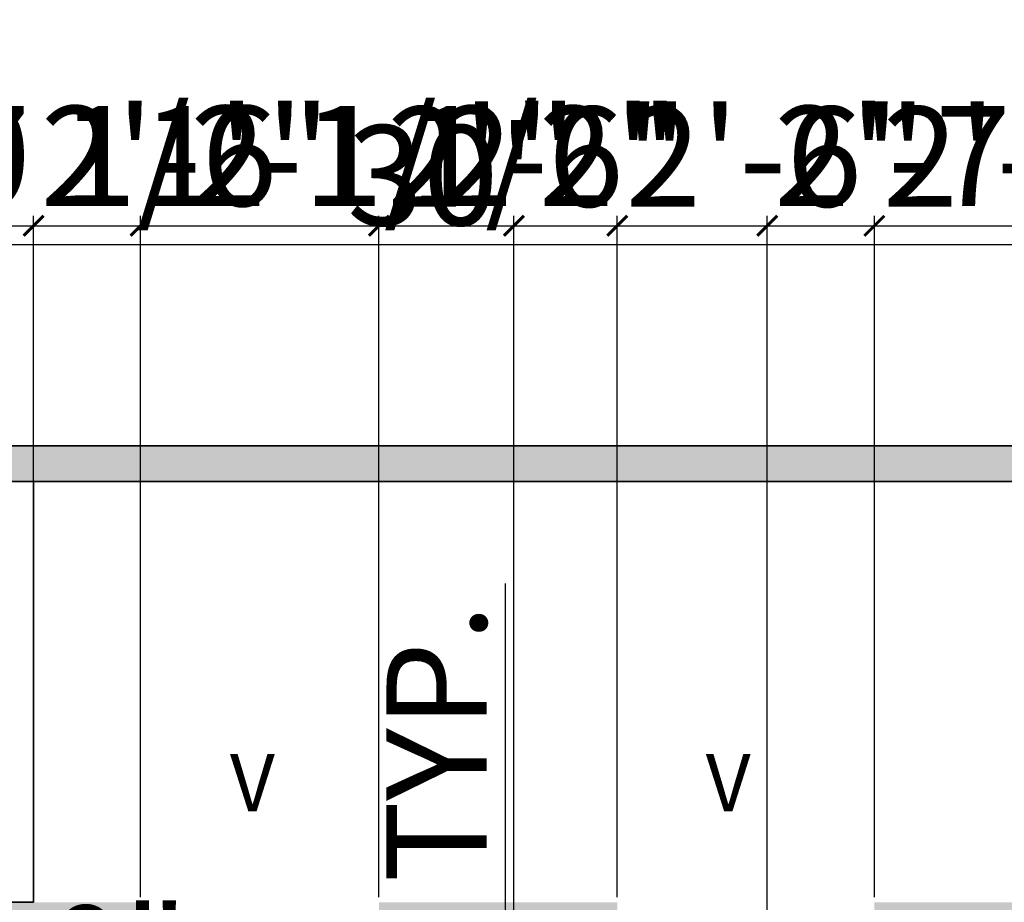
# Model space of a CAD drawing. Units: inches. Extents: x 1763 to 2368, y 1500 to 2097.
# Tile 12 of 24: x 1956 to 2079, y 1986 to 2097. Entities that reach past the tile are written whole.
import ezdxf

# ---------------------------------------------------------------- set-up
doc = ezdxf.new("R2010")
doc.units = ezdxf.units.IN
for name, color, linetype, lineweight in [('A-ANNO-DIMS', 2, 'Continuous', 18), ('A-ANNO-TEXT', 7, 'Continuous', 18), ('A-WALL', 7, 'Continuous', 35), ('A-WALL-PATT', 7, 'Continuous', 13)]:
    doc.layers.add(name, color=color, linetype=linetype, lineweight=lineweight)
doc.styles.get("Standard").update_dxf_attribs({"font": 'arial.ttf'})
doc.dimstyles.new('ISO-25', dxfattribs={"dimtxt": 12.5, "dimasz": 2.5, "dimexe": 1.25, "dimexo": 0.625, "dimtad": 1, "dimdec": 0, "dimlunit": 4, "dimtxsty": 'Standard', "dimblk": 'ARCHTICK', "dimcen": 2.5, "dimclrd": 3, "dimclrt": 4, "dimadec": 0, "dimazin": 0, "dimtfac": 1, "dimtdec": 0, "dimtmove": 0, "dimatfit": 3, "dimfxl": 1, "dimarcsym": 0})

# ---------------------------------------------------------------- blocks, each defined once
blk = doc.blocks.new('_ArchTick')
at = {"color": 0, "linetype": 'ByBlock', "const_width": 0.15}
blk.add_lwpolyline([(-0.5, -0.5), (0.5, 0.5)], dxfattribs=at)
blk = doc.blocks.new('*D21')
at = {"layer": 'A-ANNO-DIMS', "color": 0, "lineweight": -2, "transparency": 16777216}
for p, q in [((1829.09, 2043.9), (1829.09, 2069.68)), ((2189.09, 2043.9), (2189.09, 2069.68)), ((1829.09, 2068.43), (2189.09, 2068.43))]:
    blk.add_line(p, q, dxfattribs=at)
at = {"layer": 'Defpoints', "color": 0, "transparency": 16777216}
for p in [(2189.09, 2068.43), (1829.09, 2043.27), (2189.09, 2043.27)]:
    blk.add_point(p, dxfattribs=at)
at = {"layer": 'A-ANNO-DIMS', "color": 0, "lineweight": -2, "transparency": 16777216, "xscale": 2.5, "yscale": 2.5, "zscale": 2.5, "rotation": 180}
blk.add_blockref('_ArchTick', (1829.09, 2068.43), dxfattribs=at)
at = {"layer": 'A-ANNO-DIMS', "color": 0, "lineweight": -2, "transparency": 16777216, "xscale": 2.5, "yscale": 2.5, "zscale": 2.5}
blk.add_blockref('_ArchTick', (2189.09, 2068.43), dxfattribs=at)
at = {"layer": 'A-ANNO-DIMS', "color": 0, "transparency": 16777216, "insert": (2009.09, 2075.45), "char_height": 12.5, "attachment_point": 5}
blk.add_mtext("30'", dxfattribs=at)
blk = doc.blocks.new('*D35')
at = {"layer": 'A-ANNO-DIMS', "color": 0, "lineweight": -2, "transparency": 16777216}
for p, q in [((1889.68, 1972.15), (1889.68, 1969.72)), ((1901.68, 1972.15), (1901.68, 1969.72))]:
    blk.add_line(p, q, dxfattribs=at)
at = {"layer": 'A-ANNO-DIMS', "color": 3, "lineweight": -2, "transparency": 16777216}
for p, q in [((1889.68, 1970.97), (1901.68, 1970.97)), ((1901.68, 1970.97), (1977.79, 1970.97))]:
    blk.add_line(p, q, dxfattribs=at)
at = {"layer": 'Defpoints', "color": 0, "transparency": 16777216}
for p in [(1889.68, 1972.77), (1901.68, 1972.77), (1901.68, 1970.97)]:
    blk.add_point(p, dxfattribs=at)
at = {"layer": 'A-ANNO-DIMS', "color": 3, "lineweight": -2, "transparency": 16777216, "xscale": 2.5, "yscale": 2.5, "zscale": 2.5, "rotation": 180}
blk.add_blockref('_ArchTick', (1889.68, 1970.97), dxfattribs=at)
at = {"layer": 'A-ANNO-DIMS', "color": 3, "lineweight": -2, "transparency": 16777216, "xscale": 2.5, "yscale": 2.5, "zscale": 2.5}
blk.add_blockref('_ArchTick', (1901.68, 1970.97), dxfattribs=at)
at = {"layer": 'A-ANNO-DIMS', "color": 4, "transparency": 16777216, "insert": (1940.99, 1977.98), "char_height": 12.5, "attachment_point": 5}
blk.add_mtext('TAP 1\'-0"', dxfattribs=at)
blk = doc.blocks.new('*D37')
at = {"layer": 'A-ANNO-DIMS', "color": 3, "lineweight": -2, "transparency": 16777216}
for p, q in [((2017.06, 1907.01), (2017.06, 2026.09)), ((2017.06, 1900.14), (2017.06, 1907.01))]:
    blk.add_line(p, q, dxfattribs=at)
at = {"layer": 'A-ANNO-DIMS', "color": 0, "lineweight": -2, "transparency": 16777216}
for p, q in [((2017.47, 1907.01), (2015.81, 1907.01)), ((2017.47, 1900.14), (2015.81, 1900.14))]:
    blk.add_line(p, q, dxfattribs=at)
at = {"layer": 'Defpoints', "color": 0, "transparency": 16777216}
for p in [(2017.06, 1907.01), (2018.09, 1907.01), (2018.09, 1900.14)]:
    blk.add_point(p, dxfattribs=at)
at = {"layer": 'A-ANNO-DIMS', "color": 3, "lineweight": -2, "transparency": 16777216, "xscale": 2.5, "yscale": 2.5, "zscale": 2.5}
for p, rotation in [((2017.06, 1907.01), 90), ((2017.06, 1900.14), 270)]:
    blk.add_blockref('_ArchTick', p, dxfattribs=dict(at, rotation=rotation))
at = {"layer": 'A-ANNO-DIMS', "color": 4, "transparency": 16777216, "insert": (2010.05, 1967.8), "char_height": 12.5, "attachment_point": 5, "rotation": 90}
blk.add_mtext('TAP 0\'-7" TYP.', dxfattribs=at)
blk = doc.blocks.new('*D58')
at = {"layer": 'A-ANNO-DIMS', "color": 0, "lineweight": -2, "transparency": 16777216}
for p, q in [((1871.68, 1635.9), (1871.68, 2072.02)), ((1927.07, 1635.9), (1927.07, 2072.02))]:
    blk.add_line(p, q, dxfattribs=at)
at = {"layer": 'A-ANNO-DIMS', "color": 3, "lineweight": -2, "transparency": 16777216}
for p, q in [((1871.68, 2070.77), (1927.07, 2070.77)), ((1927.07, 2070.77), (1993.68, 2070.77))]:
    blk.add_line(p, q, dxfattribs=at)
at = {"layer": 'Defpoints', "color": 0, "transparency": 16777216}
for p in [(1927.07, 2070.77), (1871.68, 1635.27), (1927.07, 1635.27)]:
    blk.add_point(p, dxfattribs=at)
at = {"layer": 'A-ANNO-DIMS', "color": 3, "lineweight": -2, "transparency": 16777216, "xscale": 2.5, "yscale": 2.5, "zscale": 2.5, "rotation": 180}
blk.add_blockref('_ArchTick', (1871.68, 2070.77), dxfattribs=at)
at = {"layer": 'A-ANNO-DIMS', "color": 3, "lineweight": -2, "transparency": 16777216, "xscale": 2.5, "yscale": 2.5, "zscale": 2.5}
blk.add_blockref('_ArchTick', (1927.07, 2070.77), dxfattribs=at)
at = {"layer": 'A-ANNO-DIMS', "color": 4, "transparency": 16777216, "insert": (1961.63, 2077.86), "char_height": 12.5, "attachment_point": 5}
blk.add_mtext('4\'-7 1/2"', dxfattribs=at)
blk = doc.blocks.new('*D66')
at = {"layer": 'A-ANNO-DIMS', "color": 0, "lineweight": -2, "transparency": 16777216}
for p, q in [((1927.39, 1986.9), (1927.39, 2072.02)), ((1958.09, 1986.9), (1958.09, 2072.02))]:
    blk.add_line(p, q, dxfattribs=at)
at = {"layer": 'A-ANNO-DIMS', "color": 3, "lineweight": -2, "transparency": 16777216}
for p, q in [((1927.39, 2070.77), (1958.09, 2070.77)), ((1958.09, 2070.77), (2024.41, 2070.77))]:
    blk.add_line(p, q, dxfattribs=at)
at = {"layer": 'Defpoints', "color": 0, "transparency": 16777216}
for p in [(1958.09, 2070.77), (1927.39, 1986.27), (1958.09, 1986.27)]:
    blk.add_point(p, dxfattribs=at)
at = {"layer": 'A-ANNO-DIMS', "color": 3, "lineweight": -2, "transparency": 16777216, "xscale": 2.5, "yscale": 2.5, "zscale": 2.5, "rotation": 180}
blk.add_blockref('_ArchTick', (1927.39, 2070.77), dxfattribs=at)
at = {"layer": 'A-ANNO-DIMS', "color": 3, "lineweight": -2, "transparency": 16777216, "xscale": 2.5, "yscale": 2.5, "zscale": 2.5}
blk.add_blockref('_ArchTick', (1958.09, 2070.77), dxfattribs=at)
at = {"layer": 'A-ANNO-DIMS', "color": 4, "transparency": 16777216, "insert": (1992.5, 2077.86), "char_height": 12.5, "attachment_point": 5}
blk.add_mtext('2\'-6 1/2"', dxfattribs=at)
blk = doc.blocks.new('*D67')
at = {"layer": 'A-ANNO-DIMS', "color": 0, "lineweight": -2, "transparency": 16777216}
for p, q in [((1890.93, 1986.9), (1890.93, 2072.02)), ((1927.39, 1986.9), (1927.39, 2072.02))]:
    blk.add_line(p, q, dxfattribs=at)
at = {"layer": 'A-ANNO-DIMS', "color": 3, "lineweight": -2, "transparency": 16777216}
for p, q in [((1890.93, 2070.77), (1927.39, 2070.77)), ((1927.39, 2070.77), (1993.49, 2070.77))]:
    blk.add_line(p, q, dxfattribs=at)
at = {"layer": 'Defpoints', "color": 0, "transparency": 16777216}
for p in [(1927.39, 2070.77), (1890.93, 1986.27), (1927.39, 1986.27)]:
    blk.add_point(p, dxfattribs=at)
at = {"layer": 'A-ANNO-DIMS', "color": 3, "lineweight": -2, "transparency": 16777216, "xscale": 2.5, "yscale": 2.5, "zscale": 2.5, "rotation": 180}
blk.add_blockref('_ArchTick', (1890.93, 2070.77), dxfattribs=at)
at = {"layer": 'A-ANNO-DIMS', "color": 3, "lineweight": -2, "transparency": 16777216, "xscale": 2.5, "yscale": 2.5, "zscale": 2.5}
blk.add_blockref('_ArchTick', (1927.39, 2070.77), dxfattribs=at)
at = {"layer": 'A-ANNO-DIMS', "color": 4, "transparency": 16777216, "insert": (1961.69, 2077.87), "char_height": 12.5, "attachment_point": 5}
blk.add_mtext('3\'-0 1/2"', dxfattribs=at)
blk = doc.blocks.new('*D72')
at = {"layer": 'A-ANNO-DIMS', "color": 0, "lineweight": -2, "transparency": 16777216}
for p, q in [((2018.09, 1885.9), (2018.09, 2072.02)), ((2049.74, 1885.9), (2049.74, 2072.02))]:
    blk.add_line(p, q, dxfattribs=at)
at = {"layer": 'A-ANNO-DIMS', "color": 3, "lineweight": -2, "transparency": 16777216}
for p, q in [((2018.09, 2070.77), (2049.74, 2070.77)), ((2049.74, 2070.77), (2116.06, 2070.77))]:
    blk.add_line(p, q, dxfattribs=at)
at = {"layer": 'Defpoints', "color": 0, "transparency": 16777216}
for p in [(2049.74, 2070.77), (2018.09, 1885.27), (2049.74, 1885.27)]:
    blk.add_point(p, dxfattribs=at)
at = {"layer": 'A-ANNO-DIMS', "color": 3, "lineweight": -2, "transparency": 16777216, "xscale": 2.5, "yscale": 2.5, "zscale": 2.5, "rotation": 180}
blk.add_blockref('_ArchTick', (2018.09, 2070.77), dxfattribs=at)
at = {"layer": 'A-ANNO-DIMS', "color": 3, "lineweight": -2, "transparency": 16777216, "xscale": 2.5, "yscale": 2.5, "zscale": 2.5}
blk.add_blockref('_ArchTick', (2049.74, 2070.77), dxfattribs=at)
at = {"layer": 'A-ANNO-DIMS', "color": 4, "transparency": 16777216, "insert": (2084.15, 2077.86), "char_height": 12.5, "attachment_point": 5}
blk.add_mtext('2\'-7 1/2"', dxfattribs=at)
blk = doc.blocks.new('*D73')
at = {"layer": 'A-ANNO-DIMS', "color": 0, "lineweight": -2, "transparency": 16777216}
for p, q in [((1958.09, 1986.9), (1958.09, 2072.02)), ((1971.46, 1986.9), (1971.46, 2072.02))]:
    blk.add_line(p, q, dxfattribs=at)
at = {"layer": 'A-ANNO-DIMS', "color": 3, "lineweight": -2, "transparency": 16777216}
for p, q in [((1958.09, 2070.77), (1971.46, 2070.77)), ((1971.46, 2070.77), (2036.38, 2070.77))]:
    blk.add_line(p, q, dxfattribs=at)
at = {"layer": 'Defpoints', "color": 0, "transparency": 16777216}
for p in [(1971.46, 2070.77), (1958.09, 1986.27), (1971.46, 1986.27)]:
    blk.add_point(p, dxfattribs=at)
at = {"layer": 'A-ANNO-DIMS', "color": 3, "lineweight": -2, "transparency": 16777216, "xscale": 2.5, "yscale": 2.5, "zscale": 2.5, "rotation": 180}
blk.add_blockref('_ArchTick', (1958.09, 2070.77), dxfattribs=at)
at = {"layer": 'A-ANNO-DIMS', "color": 3, "lineweight": -2, "transparency": 16777216, "xscale": 2.5, "yscale": 2.5, "zscale": 2.5}
blk.add_blockref('_ArchTick', (1971.46, 2070.77), dxfattribs=at)
at = {"layer": 'A-ANNO-DIMS', "color": 4, "transparency": 16777216, "insert": (2005.17, 2077.86), "char_height": 12.5, "attachment_point": 5}
blk.add_mtext('1\'-1 1/2"', dxfattribs=at)
blk = doc.blocks.new('*D74')
at = {"layer": 'A-ANNO-DIMS', "color": 0, "lineweight": -2, "transparency": 16777216}
for p, q in [((1971.46, 1986.9), (1971.46, 2072.02)), ((2001.23, 1986.9), (2001.23, 2072.02))]:
    blk.add_line(p, q, dxfattribs=at)
at = {"layer": 'A-ANNO-DIMS', "color": 3, "lineweight": -2, "transparency": 16777216}
for p, q in [((1971.46, 2070.77), (2001.23, 2070.77)), ((2001.23, 2070.77), (2038.42, 2070.77))]:
    blk.add_line(p, q, dxfattribs=at)
at = {"layer": 'Defpoints', "color": 0, "transparency": 16777216}
for p in [(2001.23, 2070.77), (1971.46, 1986.27), (2001.23, 1986.27)]:
    blk.add_point(p, dxfattribs=at)
at = {"layer": 'A-ANNO-DIMS', "color": 3, "lineweight": -2, "transparency": 16777216, "xscale": 2.5, "yscale": 2.5, "zscale": 2.5, "rotation": 180}
blk.add_blockref('_ArchTick', (1971.46, 2070.77), dxfattribs=at)
at = {"layer": 'A-ANNO-DIMS', "color": 3, "lineweight": -2, "transparency": 16777216, "xscale": 2.5, "yscale": 2.5, "zscale": 2.5}
blk.add_blockref('_ArchTick', (2001.23, 2070.77), dxfattribs=at)
at = {"layer": 'A-ANNO-DIMS', "color": 4, "transparency": 16777216, "insert": (2021.08, 2077.78), "char_height": 12.5, "attachment_point": 5}
blk.add_mtext('2\'-6"', dxfattribs=at)
blk = doc.blocks.new('*D75')
at = {"layer": 'A-ANNO-DIMS', "color": 0, "lineweight": -2, "transparency": 16777216}
for p, q in [((2001.23, 1986.9), (2001.23, 2072.02)), ((2031.02, 1986.9), (2031.02, 2072.02))]:
    blk.add_line(p, q, dxfattribs=at)
at = {"layer": 'A-ANNO-DIMS', "color": 3, "lineweight": -2, "transparency": 16777216}
for p, q in [((2001.23, 2070.77), (2031.02, 2070.77)), ((2031.02, 2070.77), (2068.21, 2070.77))]:
    blk.add_line(p, q, dxfattribs=at)
at = {"layer": 'Defpoints', "color": 0, "transparency": 16777216}
for p in [(2031.02, 2070.77), (2001.23, 1986.27), (2031.02, 1986.27)]:
    blk.add_point(p, dxfattribs=at)
at = {"layer": 'A-ANNO-DIMS', "color": 3, "lineweight": -2, "transparency": 16777216, "xscale": 2.5, "yscale": 2.5, "zscale": 2.5, "rotation": 180}
blk.add_blockref('_ArchTick', (2001.23, 2070.77), dxfattribs=at)
at = {"layer": 'A-ANNO-DIMS', "color": 3, "lineweight": -2, "transparency": 16777216, "xscale": 2.5, "yscale": 2.5, "zscale": 2.5}
blk.add_blockref('_ArchTick', (2031.02, 2070.77), dxfattribs=at)
at = {"layer": 'A-ANNO-DIMS', "color": 4, "transparency": 16777216, "insert": (2050.86, 2077.78), "char_height": 12.5, "attachment_point": 5}
blk.add_mtext('2\'-6"', dxfattribs=at)
blk = doc.blocks.new('*D76')
at = {"layer": 'A-ANNO-DIMS', "color": 0, "lineweight": -2, "transparency": 16777216}
for p, q in [((2031.02, 1986.9), (2031.02, 2072.02)), ((2063.14, 1986.9), (2063.14, 2072.02))]:
    blk.add_line(p, q, dxfattribs=at)
at = {"layer": 'A-ANNO-DIMS', "color": 3, "lineweight": -2, "transparency": 16777216}
for p, q in [((2031.02, 2070.77), (2063.14, 2070.77)), ((2063.14, 2070.77), (2100.33, 2070.77))]:
    blk.add_line(p, q, dxfattribs=at)
at = {"layer": 'Defpoints', "color": 0, "transparency": 16777216}
for p in [(2063.14, 2070.77), (2031.02, 1986.27), (2063.14, 1986.27)]:
    blk.add_point(p, dxfattribs=at)
at = {"layer": 'A-ANNO-DIMS', "color": 3, "lineweight": -2, "transparency": 16777216, "xscale": 2.5, "yscale": 2.5, "zscale": 2.5, "rotation": 180}
blk.add_blockref('_ArchTick', (2031.02, 2070.77), dxfattribs=at)
at = {"layer": 'A-ANNO-DIMS', "color": 3, "lineweight": -2, "transparency": 16777216, "xscale": 2.5, "yscale": 2.5, "zscale": 2.5}
blk.add_blockref('_ArchTick', (2063.14, 2070.77), dxfattribs=at)
at = {"layer": 'A-ANNO-DIMS', "color": 4, "transparency": 16777216, "insert": (2082.99, 2077.78), "char_height": 12.5, "attachment_point": 5}
blk.add_mtext('2\'-8"', dxfattribs=at)
blk = doc.blocks.new('*D84')
at = {"layer": 'A-ANNO-DIMS', "color": 0, "lineweight": -2, "transparency": 16777216}
for p, q in [((1829.09, 2043.9), (1829.09, 2072.02)), ((1958.09, 2039.45), (1958.09, 2072.02))]:
    blk.add_line(p, q, dxfattribs=at)
at = {"layer": 'A-ANNO-DIMS', "color": 3, "lineweight": -2, "transparency": 16777216}
blk.add_line((1829.09, 2070.77), (1958.09, 2070.77), dxfattribs=at)
at = {"layer": 'Defpoints', "color": 0, "transparency": 16777216}
for p in [(1958.09, 2070.77), (1829.09, 2043.27), (1958.09, 2038.83)]:
    blk.add_point(p, dxfattribs=at)
at = {"layer": 'A-ANNO-DIMS', "color": 3, "lineweight": -2, "transparency": 16777216, "xscale": 2.5, "yscale": 2.5, "zscale": 2.5, "rotation": 180}
blk.add_blockref('_ArchTick', (1829.09, 2070.77), dxfattribs=at)
at = {"layer": 'A-ANNO-DIMS', "color": 3, "lineweight": -2, "transparency": 16777216, "xscale": 2.5, "yscale": 2.5, "zscale": 2.5}
blk.add_blockref('_ArchTick', (1958.09, 2070.77), dxfattribs=at)
at = {"layer": 'A-ANNO-DIMS', "color": 4, "transparency": 16777216, "insert": (1893.59, 2077.78), "char_height": 12.5, "attachment_point": 5}
blk.add_mtext('10\'-9"', dxfattribs=at)
blk = doc.blocks.new('*D85')
at = {"layer": 'A-ANNO-DIMS', "color": 0, "lineweight": -2, "transparency": 16777216}
for p, q in [((1957.47, 1986.27), (1787.6, 1986.27)), ((1958.51, 1880.27), (1787.6, 1880.27))]:
    blk.add_line(p, q, dxfattribs=at)
at = {"layer": 'A-ANNO-DIMS', "color": 3, "lineweight": -2, "transparency": 16777216}
blk.add_line((1788.85, 1986.27), (1788.85, 1880.27), dxfattribs=at)
at = {"layer": 'Defpoints', "color": 0, "transparency": 16777216}
for p in [(1958.09, 1986.27), (1788.85, 1880.27), (1959.13, 1880.27)]:
    blk.add_point(p, dxfattribs=at)
at = {"layer": 'A-ANNO-DIMS', "color": 3, "lineweight": -2, "transparency": 16777216, "xscale": 2.5, "yscale": 2.5, "zscale": 2.5}
for p, rotation in [((1788.85, 1986.27), 90), ((1788.85, 1880.27), 270)]:
    blk.add_blockref('_ArchTick', p, dxfattribs=dict(at, rotation=rotation))
at = {"layer": 'A-ANNO-DIMS', "color": 4, "transparency": 16777216, "insert": (1781.85, 1933.27), "char_height": 12.5, "attachment_point": 5, "rotation": 90}
blk.add_mtext('8\'-10"', dxfattribs=at)

msp = doc.modelspace()

# ---------------------------------------------------------------- hatches: boundary and pattern name
at = {"layer": 'A-WALL-PATT'}
h = msp.add_hatch(color=256, dxfattribs=at)
h.dxf.hatch_style = 1
h.paths.add_polyline_path([(1838.09, 2034.27), (1838.09, 2043.27), (1829.09, 2043.27), (1829.09, 1953.39), (1838.09, 1953.39)])
h.paths.add_polyline_path([(1838.09, 1913.1), (1829.09, 1913.1), (1829.09, 1862.2), (1838.09, 1862.2)])
h.paths.add_polyline_path([(1838.09, 1825.59), (1829.09, 1825.59), (1829.09, 1738.64), (1838.09, 1738.64)])
h.paths.add_polyline_path([(1895.59, 1885.27), (1838.09, 1885.27), (1838.09, 1880.27), (1895.59, 1880.27)])
h.paths.add_polyline_path([(1857.39, 1784.27), (1838.09, 1784.27), (1838.09, 1779.27), (1857.39, 1779.27)])
h.paths.add_polyline_path([(1958.09, 1981.27), (1971.46, 1981.27), (1971.46, 1986.27), (1968.57, 1986.27), (1958.09, 1986.27), (1953.09, 1986.27), (1927.39, 1986.27), (1927.39, 1981.27), (1953.09, 1981.27), (1953.09, 1885.27), (1932.01, 1885.27), (1932.01, 1880.27), (1959.13, 1880.27), (1959.13, 1883.74), (1959.13, 1885.27), (1958.09, 1885.27)])
h.paths.add_polyline_path([(2018.09, 1981.27), (2031.02, 1981.27), (2031.02, 1986.27), (2018.09, 1986.27), (2013.09, 1986.27), (2001.23, 1986.27), (2001.23, 1981.27), (2013.09, 1981.27), (2013.09, 1885.27), (1982.18, 1885.27, -0.016629), (1982.23, 1883.74), (1982.23, 1880.27), (2049.69, 1880.27), (2049.69, 1883.74, -0.016629), (2049.74, 1885.27), (2018.09, 1885.27)])
h.paths.add_polyline_path([(2083.09, 1981.27), (2120.61, 1981.27), (2120.61, 1986.27), (2083.09, 1986.27), (2078.09, 1986.27), (2063.14, 1986.27), (2063.14, 1981.27), (2078.09, 1981.27), (2078.09, 1885.27), (2072.78, 1885.27), (2072.78, 1883.74), (2072.78, 1880.27), (2078.09, 1880.27), (2078.09, 1866.87), (2081.56, 1866.87, -0.016629), (2083.09, 1866.82)])
h.paths.add_polyline_path([(1871.68, 1635.27), (1838.09, 1635.27), (1838.09, 1626.27), (1871.68, 1626.27)], flags=17)
h.paths.add_polyline_path([(2100.58, 1688.27), (2060.09, 1688.27), (2060.09, 1679.27), (2100.58, 1679.27)], flags=17)
h.paths.add_polyline_path([(2180.09, 1688.27), (2148.74, 1688.27), (2148.74, 1679.27), (2180.09, 1679.27)], flags=17)
h.paths.add_polyline_path([(2189.09, 1746.22), (2180.09, 1746.22), (2180.09, 1743.42), (2180.12, 1743.42), (2180.12, 1726.72), (2180.09, 1572.27), (2034.91, 1572.27), (2034.91, 1565.6), (2034.91, 1563.27), (2189.09, 1563.27)])
h.paths.add_polyline_path([(2060.09, 1802.35, -0.016629), (2058.56, 1802.3), (2055.09, 1802.3), (2055.09, 1635.27), (2042.48, 1635.27), (2042.48, 1629.74), (2042.48, 1626.27), (2055.09, 1626.27), (2055.09, 1599.27), (2040.27, 1599.27), (2040.27, 1590.27), (2060.09, 1590.27)])
h.paths.add_polyline_path([(2019.39, 1629.74, -0.060569), (2020.06, 1635.27), (1995.09, 1635.27), (1990.09, 1635.27), (1927.07, 1635.27), (1927.07, 1626.27), (1990.09, 1626.27), (1990.09, 1590.27), (1995.09, 1590.27), (2005.2, 1590.27), (2005.2, 1599.27), (1995.09, 1599.27), (1995.09, 1626.27), (2019.39, 1626.27)])
edge = h.paths.add_edge_path()
edge.add_line((2180.09, 1837.27), (2167.2, 1837.27))
edge.add_spline(control_points=[(2167.2, 1837.27), (2167.19, 1837.27), (2167.18, 1837.27), (2167.18, 1837.27)], knot_values=[168.955493, 168.955493, 168.955493, 168.955493, 169.065871, 169.065871, 169.065871, 169.065871], degree=3, periodic=0)
edge.add_spline(control_points=[(2167.18, 1837.27), (2166.56, 1837.38), (2166.33, 1846.16), (2165.71, 1846.24)], knot_values=[159.864705, 159.864705, 159.864705, 159.864705, 168.955493, 168.955493, 168.955493, 168.955493], degree=3, periodic=0)
edge.add_line((2167.12, 1837.27), (2163.16, 1837.27))
edge.add_spline(control_points=[(2163.16, 1837.27), (2163.16, 1837.27), (2163.16, 1837.27), (2163.15, 1837.27)], knot_values=[150.537172, 150.537172, 150.537172, 150.537172, 150.553797, 150.553797, 150.553797, 150.553797], degree=3, periodic=0)
edge.add_spline(control_points=[(2163.15, 1837.27), (2162.29, 1837.29), (2161.59, 1846.23), (2160.88, 1846.24)], knot_values=[141.293426, 141.293426, 141.293426, 141.293426, 150.537172, 150.537172, 150.537172, 150.537172], degree=3, periodic=0)
edge.add_line((2163.08, 1837.27), (2158.7, 1837.27))
edge.add_spline(control_points=[(2158.7, 1837.27), (2158.7, 1837.27), (2158.7, 1837.27), (2158.7, 1837.27)], knot_values=[132.033544, 132.033544, 132.033544, 132.033544, 132.049151, 132.049151, 132.049151, 132.049151], degree=3, periodic=0)
edge.add_spline(control_points=[(2158.7, 1837.27), (2157.97, 1837.29), (2157.26, 1846.23), (2156.39, 1846.24)], knot_values=[122.786021, 122.786021, 122.786021, 122.786021, 132.033544, 132.033544, 132.033544, 132.033544], degree=3, periodic=0)
edge.add_line((2158.63, 1837.27), (2153.84, 1837.27))
edge.add_spline(control_points=[(2153.84, 1837.27), (2153.83, 1837.27), (2153.82, 1837.27), (2153.82, 1837.27)], knot_values=[113.451585, 113.451585, 113.451585, 113.451585, 113.562103, 113.562103, 113.562103, 113.562103], degree=3, periodic=0)
edge.add_spline(control_points=[(2153.82, 1837.27), (2153.17, 1837.38), (2152.88, 1846.19), (2152.4, 1846.24)], knot_values=[0, 0, 0, 0, 9.081854, 9.081854, 9.081854, 9.081854], degree=3, periodic=0)
edge.add_line((2153.76, 1837.27), (2150.39, 1837.27))
edge.add_spline(control_points=[(2150.39, 1837.27), (2150.38, 1837.27), (2150.37, 1837.27), (2150.36, 1837.27)], knot_values=[95.069382, 95.069382, 95.069382, 95.069382, 95.17519, 95.17519, 95.17519, 95.17519], degree=3, periodic=0)
edge.add_spline(control_points=[(2150.36, 1837.27), (2149.49, 1837.37), (2148.42, 1846.19), (2147.59, 1846.24)], knot_values=[85.824599, 85.824599, 85.824599, 85.824599, 95.069382, 95.069382, 95.069382, 95.069382], degree=3, periodic=0)
edge.add_line((2150.29, 1837.27), (2145.43, 1837.27))
edge.add_spline(control_points=[(2145.43, 1837.27), (2145.43, 1837.27), (2145.42, 1837.27), (2145.42, 1837.27)], knot_values=[76.505559, 76.505559, 76.505559, 76.505559, 76.547811, 76.547811, 76.547811, 76.547811], degree=3, periodic=0)
edge.add_spline(control_points=[(2145.42, 1837.27), (2144.68, 1837.31), (2143.8, 1846.19), (2142.95, 1846.24)], knot_values=[67.23945, 67.23945, 67.23945, 67.23945, 76.505559, 76.505559, 76.505559, 76.505559], degree=3, periodic=0)
edge.add_line((2145.35, 1837.27), (2134.57, 1837.27))
edge.add_spline(control_points=[(2134.57, 1837.27), (2134.57, 1837.27), (2134.56, 1837.27), (2134.56, 1837.27)], knot_values=[39.001463, 39.001463, 39.001463, 39.001463, 39.045107, 39.045107, 39.045107, 39.045107], degree=3, periodic=0)
edge.add_spline(control_points=[(2134.56, 1837.27), (2133.87, 1837.31), (2133.4, 1845.85), (2132.33, 1846.24)], knot_values=[29.79778, 29.79778, 29.79778, 29.79778, 39.001463, 39.001463, 39.001463, 39.001463], degree=3, periodic=0)
edge.add_line((2134.5, 1837.27), (2128.08, 1837.27))
edge.add_spline(control_points=[(2128.08, 1837.27), (2128.03, 1837.26), (2127.98, 1837.26), (2127.93, 1837.27)], knot_values=[19.482067, 19.482067, 19.482067, 19.482067, 19.869396, 19.869396, 19.869396, 19.869396], degree=3, periodic=0)
edge.add_spline(control_points=[(2125.01, 1846.24), (2126.16, 1844.66), (2126.82, 1837.57), (2127.93, 1837.27)], knot_values=[10.389805, 10.389805, 10.389805, 10.389805, 19.482067, 19.482067, 19.482067, 19.482067], degree=3, periodic=0)
edge.add_line((2127.93, 1837.27), (2083.09, 1837.27))
edge.add_line((2083.09, 1837.27), (2083.09, 1843.77))
edge.add_line((2083.09, 1843.77), (2081.56, 1843.77))
edge.add_line((2081.56, 1843.77), (2078.09, 1843.77))
edge.add_line((2078.09, 1843.77), (2078.09, 1837.27))
edge.add_line((2078.09, 1837.27), (2055.09, 1837.27))
edge.add_line((2055.09, 1837.27), (2055.09, 1825.4))
edge.add_line((2055.09, 1825.4), (2058.56, 1825.4))
edge.add_line((2058.56, 1825.4), (2060.09, 1825.4))
edge.add_line((2060.09, 1825.4), (2060.09, 1832.27))
edge.add_line((2060.09, 1832.27), (2122.44, 1832.27))
edge.add_spline(control_points=[(2122.44, 1832.27), (2122.73, 1832.58), (2123.01, 1832.62), (2123.28, 1832.27)], knot_values=[5.972033, 5.972033, 5.972033, 5.972033, 8.057258, 8.057258, 8.057258, 8.057258], degree=3, periodic=0)
edge.add_line((2123.28, 1832.27), (2137.95, 1832.27))
edge.add_spline(control_points=[(2137.95, 1832.27), (2137.96, 1832.27), (2137.97, 1832.27), (2137.98, 1832.27)], knot_values=[53.926862, 53.926862, 53.926862, 53.926862, 54.030075, 54.030075, 54.030075, 54.030075], degree=3, periodic=0)
edge.add_spline(control_points=[(2139.72, 1825.02), (2139.28, 1825.06), (2138.67, 1832.18), (2137.98, 1832.27)], knot_values=[54.030075, 54.030075, 54.030075, 54.030075, 61.445194, 61.445194, 61.445194, 61.445194], degree=3, periodic=0)
edge.add_line((2138.05, 1832.27), (2140.96, 1832.27))
edge.add_spline(control_points=[(2140.96, 1832.27), (2140.97, 1832.27), (2140.98, 1832.27), (2140.99, 1832.27)], knot_values=[68.854182, 68.854182, 68.854182, 68.854182, 68.971237, 68.971237, 68.971237, 68.971237], degree=3, periodic=0)
edge.add_spline(control_points=[(2143.19, 1825.02), (2142.44, 1825.07), (2141.56, 1832.16), (2140.99, 1832.27)], knot_values=[68.971237, 68.971237, 68.971237, 68.971237, 76.444911, 76.444911, 76.444911, 76.444911], degree=3, periodic=0)
edge.add_line((2141.04, 1832.27), (2145.43, 1832.27))
edge.add_spline(control_points=[(2145.43, 1832.27), (2145.44, 1832.27), (2145.45, 1832.27), (2145.46, 1832.27)], knot_values=[84.039047, 84.039047, 84.039047, 84.039047, 84.124041, 84.124041, 84.124041, 84.124041], degree=3, periodic=0)
edge.add_spline(control_points=[(2148.11, 1825.02), (2147.34, 1825.02), (2146.3, 1832.19), (2145.46, 1832.27)], knot_values=[84.124041, 84.124041, 84.124041, 84.124041, 91.773891, 91.773891, 91.773891, 91.773891], degree=3, periodic=0)
edge.add_line((2145.54, 1832.27), (2150.39, 1832.27))
edge.add_spline(control_points=[(2150.39, 1832.27), (2150.42, 1832.28), (2150.45, 1832.28), (2150.47, 1832.27)], knot_values=[99.381577, 99.381577, 99.381577, 99.381577, 99.573457, 99.573457, 99.573457, 99.573457], degree=3, periodic=0)
edge.add_spline(control_points=[(2153.97, 1825.02), (2153.09, 1825.28), (2151.53, 1832.1), (2150.47, 1832.27)], knot_values=[99.573457, 99.573457, 99.573457, 99.573457, 107.218357, 107.218357, 107.218357, 107.218357], degree=3, periodic=0)
edge.add_line((2150.57, 1832.27), (2155.6, 1832.27))
edge.add_spline(control_points=[(2155.6, 1832.27), (2155.6, 1832.27), (2155.61, 1832.27), (2155.62, 1832.27)], knot_values=[114.933058, 114.933058, 114.933058, 114.933058, 115.013624, 115.013624, 115.013624, 115.013624], degree=3, periodic=0)
edge.add_spline(control_points=[(2158.28, 1825.02), (2157.4, 1825.07), (2156.25, 1832.2), (2155.62, 1832.27)], knot_values=[115.013624, 115.013624, 115.013624, 115.013624, 122.616269, 122.616269, 122.616269, 122.616269], degree=3, periodic=0)
edge.add_line((2155.68, 1832.27), (2165.19, 1832.27))
edge.add_spline(control_points=[(2165.19, 1832.27), (2165.2, 1832.27), (2165.2, 1832.27), (2165.2, 1832.27)], knot_values=[145.488477, 145.488477, 145.488477, 145.488477, 145.516379, 145.516379, 145.516379, 145.516379], degree=3, periodic=0)
edge.add_spline(control_points=[(2167.45, 1825.02), (2166.96, 1825.02), (2166.06, 1832.25), (2165.2, 1832.27)], knot_values=[145.516379, 145.516379, 145.516379, 145.516379, 153.105469, 153.105469, 153.105469, 153.105469], degree=3, periodic=0)
edge.add_line((2165.29, 1832.27), (2168.93, 1832.27))
edge.add_spline(control_points=[(2168.93, 1832.27), (2168.98, 1832.29), (2169.04, 1832.29), (2169.1, 1832.27)], knot_values=[160.517439, 160.517439, 160.517439, 160.517439, 160.939723, 160.939723, 160.939723, 160.939723], degree=3, periodic=0)
edge.add_spline(control_points=[(2171.09, 1828.64), (2170.35, 1830.37), (2169.62, 1832.09), (2169.1, 1832.27)], knot_values=[160.939723, 160.939723, 160.939723, 160.939723, 164.738835, 164.738835, 164.738835, 164.738835], degree=3, periodic=0)
edge.add_line((2169.1, 1832.27), (2180.09, 1832.27))
edge.add_line((2180.09, 1832.27), (2180.09, 1837.27))
h.paths.add_polyline_path([(2189.09, 1885.52), (2180.09, 1885.52), (2180.09, 1813.32), (2180.12, 1813.32), (2180.12, 1796.62), (2180.12, 1795.26), (2189.09, 1795.26)])
h.paths.add_polyline_path([(2180.09, 1986.27), (2166.28, 1986.27), (2166.28, 1981.27), (2180.09, 1981.27)])
h.paths.add_polyline_path([(2189.09, 2043.27), (2180.09, 2043.27), (2180.09, 2034.27), (2180.09, 1934.11), (2189.09, 1934.11)])
h.paths.add_polyline_path([(1838.09, 1681.59), (1829.09, 1681.59), (1829.09, 1563.27), (2003.86, 1563.27), (2003.86, 1565.6), (2003.86, 1572.27), (1838.09, 1572.27)])
h = msp.add_hatch(color=256, dxfattribs=at)
h.dxf.hatch_style = 1
h.paths.add_polyline_path([(2180.09, 2043.27), (1838.09, 2043.27), (1838.09, 2038.83), (2180.09, 2038.83)])

# ---------------------------------------------------------------- linework, layer by layer
at = {"layer": 'A-WALL'}
for p, q in [((1838.09, 2043.27), (2180.09, 2043.27)), ((1838.09, 2038.83), (2180.09, 2038.83)), ((1958.09, 2034.27), (1958.09, 2038.83)), ((1958.09, 2034.27), (1958.09, 2038.83)), ((1958.09, 1986.27), (1958.09, 2034.27)), ((1958.09, 1986.27), (1958.09, 2034.27)), ((1953.09, 1986.27), (1958.09, 1986.27))]:
    msp.add_line(p, q, dxfattribs=at)
msp.add_lwpolyline([(2003.86, 1563.27), (1829.09, 1563.27), (1829.09, 2043.27), (2189.09, 2043.27), (2189.09, 1563.27), (2034.91, 1563.27)], dxfattribs=at)

# ---------------------------------------------------------------- texts
at = {"layer": 'A-ANNO-TEXT'}
for p in [(1982.62, 1997.65), (2042.07, 1997.65)]:
    msp.add_text('V', height=7.15, dxfattribs=at).set_placement(p)

# ---------------------------------------------------------------- dimensions: what is measured, and where the dimension line sits
at = {"layer": 'A-ANNO-DIMS'}
for base, p1, p2, override, picture, middle in [((1927.07, 2070.77), (1871.68, 1635.27), (1927.07, 1635.27), {"dimdec": 1, "dimlfac": 1, "dimrnd": 0, "dimzin": 1, "dimdsep": 46, "dimlunit": 4, "dimfrac": 2}, '*D58', (1961.63, 2077.86)), ((1927.39, 2070.77), (1890.93, 1986.27), (1927.39, 1986.27), {"dimdec": 1, "dimlfac": 1, "dimrnd": 0, "dimzin": 1, "dimdsep": 46, "dimlunit": 4, "dimfrac": 2}, '*D67', (1961.69, 2077.87)), ((1958.09, 2070.77), (1927.39, 1986.27), (1958.09, 1986.27), {"dimdec": 1, "dimlfac": 1, "dimrnd": 0, "dimzin": 1, "dimdsep": 46, "dimlunit": 4, "dimfrac": 2}, '*D66', (1992.5, 2077.86)), ((1971.46, 2070.77), (1958.09, 1986.27), (1971.46, 1986.27), {"dimdec": 1, "dimlfac": 1, "dimrnd": 0, "dimzin": 1, "dimdsep": 46, "dimlunit": 4, "dimfrac": 2}, '*D73', (2005.17, 2077.86)), ((2049.7368, 2070.7727), (2018.0918, 1885.2727), (2049.7368, 1885.2727), {"dimdec": 1, "dimlfac": 1, "dimrnd": 0, "dimzin": 1, "dimdsep": 46, "dimlunit": 4, "dimfrac": 2}, '*D72', (2084.1459, 2077.8609)), ((1958.09, 2070.77), (1829.09, 2043.27), (1958.09, 2038.83), {"dimdec": 1, "dimlfac": 1, "dimrnd": 0, "dimzin": 1, "dimdsep": 46, "dimlunit": 4, "dimfrac": 2}, '*D84', (1893.59, 2077.78)), ((2001.23, 2070.77), (1971.46, 1986.27), (2001.23, 1986.27), {"dimdec": 1, "dimlfac": 1, "dimrnd": 0, "dimzin": 1, "dimdsep": 46, "dimlunit": 4, "dimfrac": 2}, '*D74', (2021.08, 2077.78)), ((2031.02, 2070.77), (2001.23, 1986.27), (2031.02, 1986.27), {"dimdec": 1, "dimlfac": 1, "dimrnd": 0, "dimzin": 1, "dimdsep": 46, "dimlunit": 4, "dimfrac": 2}, '*D75', (2050.86, 2077.78)), ((2063.14, 2070.77), (2031.02, 1986.27), (2063.14, 1986.27), {"dimdec": 1, "dimlfac": 1, "dimrnd": 0, "dimzin": 1, "dimdsep": 46, "dimlunit": 4, "dimfrac": 2}, '*D76', (2082.99, 2077.78)), ((2189.09, 2068.43), (1829.09, 2043.27), (2189.09, 2043.27), {"dimclrd": 0, "dimclre": 0, "dimclrt": 0}, '*D21', (2009.09, 2075.45))]:
    dim = msp.add_linear_dim(base=base, p1=p1, p2=p2, dimstyle='ISO-25', override=override, dxfattribs=at)
    dim.commit()
    dim.dimension.update_dxf_attribs({"geometry": picture, "text_midpoint": middle})
dim = msp.add_linear_dim(base=(2017.06, 1907.01), p1=(2018.09, 1900.14), p2=(2018.09, 1907.01), angle=90, text='TAP <> TYP.', dimstyle='ISO-25', override={"dimdec": 1, "dimlfac": 1, "dimrnd": 0, "dimzin": 1, "dimdsep": 46, "dimlunit": 4, "dimfrac": 2}, dxfattribs=at)
dim.commit()
dim.dimension.update_dxf_attribs({"geometry": '*D37', "text_midpoint": (2010.05, 1967.8)})
dim = msp.add_linear_dim(base=(1901.68, 1970.97), p1=(1889.68, 1972.77), p2=(1901.68, 1972.77), text='TAP <>', dimstyle='ISO-25', override={"dimdec": 1, "dimlfac": 1, "dimrnd": 0, "dimzin": 1, "dimdsep": 46, "dimlunit": 4, "dimfrac": 2}, dxfattribs=at)
dim.commit()
dim.dimension.update_dxf_attribs({"geometry": '*D35', "text_midpoint": (1940.99, 1977.98)})
dim = msp.add_linear_dim(base=(1788.85, 1880.27), p1=(1958.09, 1986.27), p2=(1959.13, 1880.27), angle=90, dimstyle='ISO-25', override={"dimdec": 1, "dimlfac": 1, "dimrnd": 0, "dimzin": 1, "dimdsep": 46, "dimlunit": 4, "dimfrac": 2}, dxfattribs=at)
dim.commit()
dim.dimension.update_dxf_attribs({"geometry": '*D85', "text_midpoint": (1781.85, 1933.27)})

doc.saveas('drawing.dxf')
